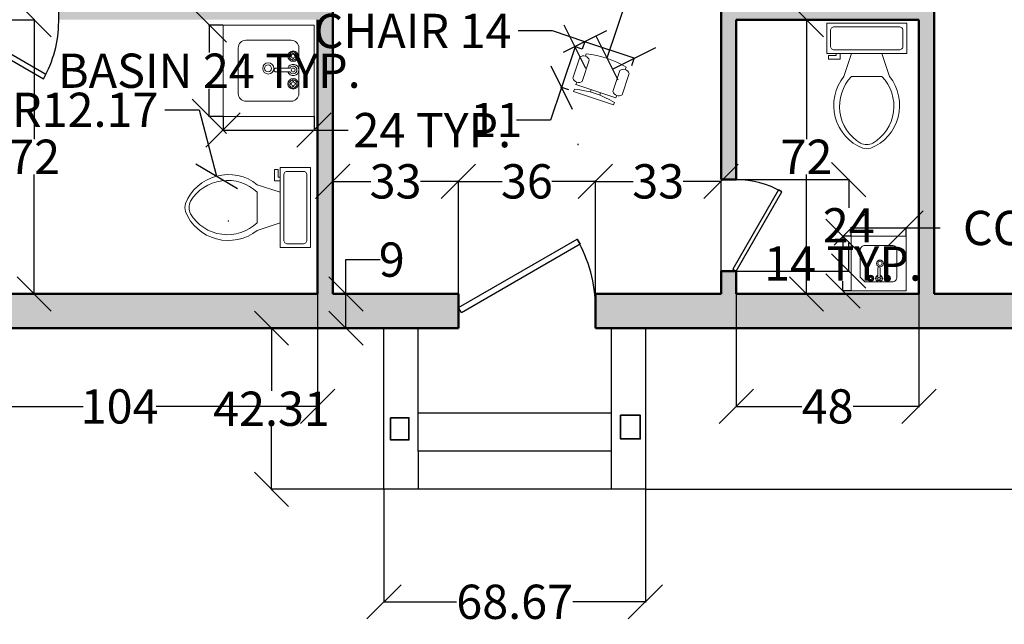
# Model space of a CAD drawing. Units: inches. Extents: x -9 to 615, y -420 to 89.
# Tile 2 of 6: x 201 to 460, y -420 to -261. Entities that reach past the tile are written whole.
import ezdxf

# ---------------------------------------------------------------- set-up
doc = ezdxf.new("R2010")
doc.units = ezdxf.units.IN
doc.header["$MEASUREMENT"] = 0
for name, color, linetype, lineweight in [('A-ANNO-DIMS', 2, 'Continuous', 18), ('A-COLS', 7, 'Continuous', 35), ('A-DOOR', 4, 'Continuous', 25), ('A-FLOR-FIXT', 9, 'Continuous', 18), ('A-FLOR-STRS', 7, 'Continuous', 25), ('A-FURN', 8, 'Continuous', 18), ('A-WALL', 7, 'Continuous', 50)]:
    doc.layers.add(name, color=color, linetype=linetype, lineweight=lineweight)
doc.layers.add('A-WALL-PATT', color=251, linetype='Continuous', lineweight=13, true_color=0x636466)
doc.styles.get("Standard").update_dxf_attribs({"font": 'arial.ttf'})
doc.dimstyles.get("Standard").update_dxf_attribs({"dimtxt": 9, "dimasz": 9, "dimexe": 0.18, "dimexo": 0.0625, "dimgap": 0.09, "dimtad": 0, "dimtih": 1, "dimtoh": 1, "dimdec": 0, "dimzin": 0, "dimdsep": 46, "dimlunit": 4, "dimtxsty": 'Standard', "dimblk": 'OBLIQUE', "dimblk2": 'OBLIQUE', "dimcen": 0.09, "dimadec": 0, "dimazin": 0, "dimtfac": 1, "dimtdec": 0, "dimtofl": 0, "dimtmove": 0, "dimatfit": 3, "dimldrblk": 'OBLIQUE', "dimfxl": 1, "dimtolj": 1, "dimtzin": 0, "dimarcsym": 0})

# ---------------------------------------------------------------- blocks, each defined once
blk = doc.blocks.new('Chair - Desk')
for p, q in [((-8.5, 0), (-8.5, -1)), ((-8.5, 0), (8.5, 0)), ((8.5, 0), (8.5, -1)), ((-8.5, -3), (-8.5, -4)), ((-8.5, -3), (8.5, -3)), ((-2, -3), (-2, -1.9355)), ((2, -1.9576), (2, -3)), ((8.5, -3), (8.5, -4)), ((-10.5, -5), (-10.5, -14)), ((-6.5, -14), (-6.5, -5)), ((6.5, -5), (6.5, -14)), ((10.5, -14), (10.5, -5)), ((-8.5, -15), (-8.5, -16)), ((8.5, -15), (8.5, -16))]:
    blk.add_line(p, q)
for centre, radius, start, end in [((0, 34.625), 36.625, 256.5803, 283.4197), ((-8.5, -6.5), 2.5, 36.8699, 143.1301), ((8.5, -6.5), 2.5, 36.8699, 143.1301), ((-8.5, -12.5), 2.5, 216.8699, 323.1301), ((8.5, -12.5), 2.5, 216.8699, 323.1301), ((0, 19.625), 36.625, 256.5803, 283.4197)]:
    blk.add_arc(centre, radius, start, end)
blk = doc.blocks.new('Toilet - top')
for p, q in [((9.5, -6), (9.5, -2)), ((-10, -8.5), (-8, -8.5)), ((-10, -9.5), (-10, -8.5)), ((-7, -9.5), (-10, -9.5)), ((-8, -8.5), (-8, -8)), ((-7, -8), (-7, -9.5)), ((-4, -8), (-6, -14)), ((4, -8), (6, -14)), ((4, -14), (-4, -14))]:
    blk.add_line(p, q)
blk.add_lwpolyline([(10.5, -8), (10.5, 0), (-10.5, 0), (-10.5, -8)], close=True)
for points in [[(-9.5, -2), (-9.5, -6)], [(8.5, -1), (-8.5, -1)], [(-8.5, -7), (8.5, -7)]]:
    blk.add_lwpolyline(points)
for centre, radius, start, end in [((-8.62, -1.88), 0.884, 81.8699, 188.1301), ((8.62, -1.88), 0.884, 351.8699, 98.1301), ((-8.62, -6.12), 0.884, 171.8699, 278.1301), ((8.62, -6.12), 0.884, 261.8699, 8.1301), ((3.52, -21.58), 12.17, 141.4691, 247.9714), ((4.2, -21.82), 11.33, 136.3677, 238.9468), ((-3.52, -21.58), 12.17, 292.0284, 38.5307), ((-4.2, -21.82), 11.33, 301.053, 43.6321), ((0, -27.88), 4, 245.7318, 294.2682), ((0, -29), 4, 254.8605, 285.1395)]:
    blk.add_arc(centre, radius, start, end)
blk = doc.blocks.new('*U12')
for p, q in [((0, 0), (0, -6)), ((40, 0), (40, -6))]:
    blk.add_line(p, q)
blk.add_lwpolyline([(0, 0), (34.64, 20), (35.52, 18.48), (0.87, -1.52)], close=True)
blk.add_arc((0, 0), 40, 0, 30)
blk = doc.blocks.new('*U13')
for p, q in [((0, 0), (0, 6)), ((40, 0), (40, 6))]:
    blk.add_line(p, q)
blk.add_lwpolyline([(0, 0), (34.64, -20), (35.52, -18.48), (0.87, 1.52)], close=True)
blk.add_arc((0, 0), 40, 330, 0)
blk = doc.blocks.new('Faucet - Bathroom top')
for p, q in [((-4.107, 0.125), (-4.375, 0.125)), ((-3.75, 0.4788), (-3.75, 0.75)), ((-3.5, 0.482), (-3.5, 0.75)), ((-3.1461, 0.125), (-2.875, 0.125)), ((3.143, 0.125), (2.875, 0.125)), ((3.5, 0.4788), (3.5, 0.75)), ((3.75, 0.482), (3.75, 0.75)), ((4.1039, 0.125), (4.375, 0.125)), ((-4.1039, -0.125), (-4.375, -0.125)), ((-3.75, -0.4821), (-3.75, -0.75)), ((-3.5, -0.4789), (-3.5, -0.75)), ((-3.143, -0.125), (-2.875, -0.125)), ((-0.5, -0.8639), (-0.5, -4.5)), ((0.5, -4.5), (0.5, -0.8631)), ((3.1461, -0.125), (2.875, -0.125)), ((3.5, -0.4821), (3.5, -0.75)), ((3.75, -0.4789), (3.75, -0.75)), ((4.107, -0.125), (4.375, -0.125))]:
    blk.add_line(p, q)
for centre, radius in [((-3.625, 0), 1.375), ((-4.625, 0), 0.2795), ((-3.625, 0), 0.5), ((-3.625, 1), 0.2795), ((-2.625, 0), 0.2795), ((0, 0), 0.5), ((3.625, 0), 1.375), ((2.625, 0), 0.2795), ((3.625, 0), 0.5), ((3.625, 1), 0.2795), ((4.625, 0), 0.2795), ((-3.625, -1), 0.2795), ((3.625, -1), 0.2795)]:
    blk.add_circle(centre, radius)
for centre, radius, start, end in [((-3.625, 0), 1, 105.2407, 164.2093), ((-3.625, 0), 1, 16.44125, 74.07887), ((0, 0), 1.5, 289.6514, 250.3603), ((0, 0), 1, 300.3431, 239.7554), ((3.625, 0), 1, 106.12, 164.0884), ((3.625, 0), 1, 16.23422, 73.90469), ((-3.625, 0), 1, 196.2342, 253.9047), ((-3.625, 0), 1, 286.12, 344.0884), ((3.625, 0), 1, 196.4413, 254.0789), ((3.625, 0), 1, 285.2407, 344.2093), ((0, -4.5), 0.5, 180, 0)]:
    blk.add_arc(centre, radius, start, end)
blk = doc.blocks.new('LAVATORY-24IN')
blk.add_lwpolyline([(0, 23.91), (0, 0), (24, 0), (24, 23.91)], close=True)
blk.add_lwpolyline([(4, 17.91), (4, 6, 0.414214), (6, 4), (18, 4, 0.414214), (20, 6), (20, 17.91, 0.414214), (18, 19.91), (6, 19.91, 0.414214)], format="xyb", close=True)
for centre, radius in [((11.41, 11.89), 1.47), ((11.39, 11.82), 0.91)]:
    blk.add_circle(centre, radius)
blk.add_blockref('Faucet - Bathroom top', (11.81, 18.42))
blk = doc.blocks.new('LAVATORY-COMPACT')
blk.add_lwpolyline([(14.42, 0), (14.42, 14.37), (0, 14.37), (0, 0)], close=True)
blk.add_lwpolyline([(12.02, 3.61), (12.02, 10.76, 0.414214), (10.82, 11.96), (3.61, 11.96, 0.414214), (2.4, 10.76), (2.4, 3.61), (3.61, 2.4), (10.82, 2.4, 0.414214)], format="xyb", close=True)
for centre, radius in [((7.57, 7.22), 0.886), ((7.57, 7.26), 0.547)]:
    blk.add_circle(centre, radius)
at = {"xscale": 0.6009252125773316, "yscale": 0.6009252125773316, "zscale": 0.6009252125773316, "rotation": 180}
blk.add_blockref('Faucet - Bathroom top', (7.32, 3.3), dxfattribs=at)
blk = doc.blocks.new('_Oblique')
at = {"color": 0, "linetype": 'ByBlock', "lineweight": -2}
blk.add_line((-0.5, -0.5), (0.5, 0.5), dxfattribs=at)
blk = doc.blocks.new('*D22')
at = {"layer": 'A-ANNO-DIMS', "color": 0, "lineweight": -2, "transparency": 16777216}
for p, q in [((254.55, -262.38), (250.83, -262.38)), ((251.01, -262.38), (251.01, -269.63)), ((251.01, -286.38), (251.01, -279.12)), ((254.55, -286.38), (250.83, -286.38))]:
    blk.add_line(p, q, dxfattribs=at)
at = {"layer": 'Defpoints', "color": 0, "transparency": 16777216}
for p in [(254.61, -262.38), (251.01, -286.38), (254.61, -286.38)]:
    blk.add_point(p, dxfattribs=at)
at = {"layer": 'A-ANNO-DIMS', "color": 0, "lineweight": -2, "transparency": 16777216, "xscale": 9, "yscale": 9, "zscale": 9}
for p, rotation in [((251.01, -262.38), 90), ((251.01, -286.38), 270)]:
    blk.add_blockref('_Oblique', p, dxfattribs=dict(at, rotation=rotation))
at = {"layer": 'A-ANNO-DIMS', "color": 0, "transparency": 16777216, "insert": (251.01, -274.38), "char_height": 9, "attachment_point": 5}
blk.add_mtext('\\A1;BASIN 24 TYP.', dxfattribs=at)
blk = doc.blocks.new('*D23')
at = {"layer": 'A-ANNO-DIMS', "color": 0, "lineweight": -2, "transparency": 16777216}
for p, q in [((254.61, -286.44), (254.61, -290.16)), ((278.52, -286.44), (278.52, -290.16)), ((254.61, -289.98), (278.52, -289.98)), ((278.52, -289.98), (287.52, -289.98))]:
    blk.add_line(p, q, dxfattribs=at)
at = {"layer": 'Defpoints', "color": 0, "transparency": 16777216}
for p in [(254.61, -286.38), (278.52, -286.38), (278.52, -289.98)]:
    blk.add_point(p, dxfattribs=at)
at = {"layer": 'A-ANNO-DIMS', "color": 0, "lineweight": -2, "transparency": 16777216, "xscale": 9, "yscale": 9, "zscale": 9, "rotation": 180}
blk.add_blockref('_Oblique', (254.61, -289.98), dxfattribs=at)
at = {"layer": 'A-ANNO-DIMS', "color": 0, "lineweight": -2, "transparency": 16777216, "xscale": 9, "yscale": 9, "zscale": 9}
blk.add_blockref('_Oblique', (278.52, -289.98), dxfattribs=at)
at = {"layer": 'A-ANNO-DIMS', "color": 0, "transparency": 16777216, "insert": (309.59, -289.98), "char_height": 9, "attachment_point": 5}
blk.add_mtext('\\A1;24 TYP.', dxfattribs=at)
blk = doc.blocks.new('*D24')
at = {"layer": 'A-ANNO-DIMS', "color": 0, "lineweight": -2, "transparency": 16777216}
for p, q in [((419.63, -317.77), (419.63, -315.49)), ((434.05, -317.77), (434.05, -315.49)), ((419.63, -315.67), (434.05, -315.67)), ((434.05, -315.67), (443.05, -315.67))]:
    blk.add_line(p, q, dxfattribs=at)
at = {"layer": 'Defpoints', "color": 0, "transparency": 16777216}
for p in [(419.63, -317.84), (434.05, -315.67), (434.05, -317.84)]:
    blk.add_point(p, dxfattribs=at)
at = {"layer": 'A-ANNO-DIMS', "color": 0, "lineweight": -2, "transparency": 16777216, "xscale": 9, "yscale": 9, "zscale": 9, "rotation": 180}
blk.add_blockref('_Oblique', (419.63, -315.67), dxfattribs=at)
at = {"layer": 'A-ANNO-DIMS', "color": 0, "lineweight": -2, "transparency": 16777216, "xscale": 9, "yscale": 9, "zscale": 9}
blk.add_blockref('_Oblique', (434.05, -315.67), dxfattribs=at)
at = {"layer": 'A-ANNO-DIMS', "color": 0, "transparency": 16777216, "insert": (518.79, -315.67), "char_height": 9, "attachment_point": 5}
blk.add_mtext('\\A1;COMPACT BASIN 14 TYP.', dxfattribs=at)
blk = doc.blocks.new('*D25')
at = {"layer": 'A-ANNO-DIMS', "color": 0, "lineweight": -2, "transparency": 16777216}
for p, q in [((419.57, -317.84), (417.29, -317.84)), ((417.47, -317.84), (417.47, -320.41)), ((417.47, -332.2), (417.47, -329.63)), ((419.57, -332.2), (417.29, -332.2))]:
    blk.add_line(p, q, dxfattribs=at)
at = {"layer": 'Defpoints', "color": 0, "transparency": 16777216}
for p in [(417.47, -317.84), (419.63, -317.84), (419.63, -332.2)]:
    blk.add_point(p, dxfattribs=at)
at = {"layer": 'A-ANNO-DIMS', "color": 0, "lineweight": -2, "transparency": 16777216, "xscale": 9, "yscale": 9, "zscale": 9}
for p, rotation in [((417.47, -317.84), 90), ((417.47, -332.2), 270)]:
    blk.add_blockref('_Oblique', p, dxfattribs=dict(at, rotation=rotation))
at = {"layer": 'A-ANNO-DIMS', "color": 0, "transparency": 16777216, "insert": (417.47, -325.02), "char_height": 9, "attachment_point": 5}
blk.add_mtext('\\A1;14 TYP.', dxfattribs=at)
blk = doc.blocks.new('*D30')
at = {"layer": 'A-ANNO-DIMS', "color": 0, "lineweight": -2, "transparency": 16777216}
for p, q in [((341.16, -263.93), (332.16, -263.93)), ((349.7, -266.78), (341.16, -263.93)), ((349.07, -268.67), (349.75, -266.61)), ((362.66, -271.11), (349.7, -266.78)), ((362.03, -272.99), (362.72, -270.94))]:
    blk.add_line(p, q, dxfattribs=at)
at = {"layer": 'Defpoints', "color": 0, "transparency": 16777216}
for p in [(349.05, -268.73), (349.7, -266.78), (362.01, -273.05)]:
    blk.add_point(p, dxfattribs=at)
at = {"layer": 'A-ANNO-DIMS', "color": 0, "lineweight": -2, "transparency": 16777216, "xscale": 9, "yscale": 9, "zscale": 9}
for p, rotation in [((349.7, -266.78), 161.5484668350482), ((362.66, -271.11), 341.5484668350483)]:
    blk.add_blockref('_Oblique', p, dxfattribs=dict(at, rotation=rotation))
at = {"layer": 'A-ANNO-DIMS', "color": 0, "transparency": 16777216, "insert": (304.39, -263.93), "char_height": 9, "attachment_point": 5}
blk.add_mtext('\\A1;CHAIR 14', dxfattribs=at)
blk = doc.blocks.new('*D31')
at = {"layer": 'A-ANNO-DIMS', "color": 0, "lineweight": -2, "transparency": 16777216}
for p, q in [((347.1, -268.08), (343.53, -278.78)), ((348.99, -268.71), (346.93, -268.02)), ((343.53, -278.78), (340.68, -287.32)), ((345.42, -279.41), (343.36, -278.72)), ((340.68, -287.32), (331.68, -287.32))]:
    blk.add_line(p, q, dxfattribs=at)
at = {"layer": 'Defpoints', "color": 0, "transparency": 16777216}
for p in [(349.05, -268.73), (343.53, -278.78), (345.48, -279.43)]:
    blk.add_point(p, dxfattribs=at)
at = {"layer": 'A-ANNO-DIMS', "color": 0, "lineweight": -2, "transparency": 16777216, "xscale": 9, "yscale": 9, "zscale": 9}
for p, rotation in [((347.1, -268.08), 71.54846683504834), ((343.53, -278.78), 251.5484668350484)]:
    blk.add_blockref('_Oblique', p, dxfattribs=dict(at, rotation=rotation))
at = {"layer": 'A-ANNO-DIMS', "color": 0, "transparency": 16777216, "insert": (326.44, -287.32), "char_height": 9, "attachment_point": 5}
blk.add_mtext('\\A1;11', dxfattribs=at)
blk = doc.blocks.new('*D42')
at = {"layer": 'A-ANNO-DIMS', "color": 0, "lineweight": -2, "transparency": 16777216}
for p, q in [((437.5, 54.02), (600.17, 54.02)), ((599.99, 54.02), (599.99, -160.45)), ((599.99, -384.29), (599.99, -169.82)), ((365.62, -384.29), (600.17, -384.29))]:
    blk.add_line(p, q, dxfattribs=at)
at = {"layer": 'Defpoints', "color": 0, "transparency": 16777216}
for p in [(437.44, 54.02), (599.99, 54.02), (365.56, -384.29)]:
    blk.add_point(p, dxfattribs=at)
at = {"layer": 'A-ANNO-DIMS', "color": 0, "lineweight": -2, "transparency": 16777216, "xscale": 9, "yscale": 9, "zscale": 9}
for p, rotation in [((599.99, 54.02), 90), ((599.99, -384.29), 270)]:
    blk.add_blockref('_Oblique', p, dxfattribs=dict(at, rotation=rotation))
at = {"layer": 'A-ANNO-DIMS', "color": 0, "transparency": 16777216, "insert": (599.99, -165.14), "char_height": 9, "attachment_point": 5}
blk.add_mtext('\\A1;438.3', dxfattribs=at)
blk = doc.blocks.new('*D50')
at = {"layer": 'A-ANNO-DIMS', "color": 0, "lineweight": -2, "transparency": 16777216}
for p, q in [((175.44, -333.04), (175.44, -362.71)), ((279.44, -333.04), (279.44, -362.71)), ((175.44, -362.53), (217.85, -362.53)), ((279.44, -362.53), (237.03, -362.53))]:
    blk.add_line(p, q, dxfattribs=at)
at = {"layer": 'Defpoints', "color": 0, "transparency": 16777216}
for p in [(175.44, -332.98), (279.44, -332.98), (175.44, -362.53)]:
    blk.add_point(p, dxfattribs=at)
at = {"layer": 'A-ANNO-DIMS', "color": 0, "lineweight": -2, "transparency": 16777216, "xscale": 9, "yscale": 9, "zscale": 9, "rotation": 180}
blk.add_blockref('_Oblique', (175.44, -362.53), dxfattribs=at)
at = {"layer": 'A-ANNO-DIMS', "color": 0, "lineweight": -2, "transparency": 16777216, "xscale": 9, "yscale": 9, "zscale": 9}
blk.add_blockref('_Oblique', (279.44, -362.53), dxfattribs=at)
at = {"layer": 'A-ANNO-DIMS', "color": 0, "transparency": 16777216, "insert": (227.44, -362.53), "char_height": 9, "attachment_point": 5}
blk.add_mtext('\\A1;104', dxfattribs=at)
blk = doc.blocks.new('*D51')
at = {"layer": 'A-ANNO-DIMS', "color": 0, "lineweight": -2, "transparency": 16777216}
for p, q in [((283.44, -332.92), (283.44, -303.25)), ((283.44, -303.43), (293.4, -303.43)), ((316.44, -303.43), (306.47, -303.43)), ((316.44, -332.92), (316.44, -303.25))]:
    blk.add_line(p, q, dxfattribs=at)
at = {"layer": 'Defpoints', "color": 0, "transparency": 16777216}
for p in [(316.44, -303.43), (283.44, -332.98), (316.44, -332.98)]:
    blk.add_point(p, dxfattribs=at)
at = {"layer": 'A-ANNO-DIMS', "color": 0, "lineweight": -2, "transparency": 16777216, "xscale": 9, "yscale": 9, "zscale": 9, "rotation": 180}
blk.add_blockref('_Oblique', (283.44, -303.43), dxfattribs=at)
at = {"layer": 'A-ANNO-DIMS', "color": 0, "lineweight": -2, "transparency": 16777216, "xscale": 9, "yscale": 9, "zscale": 9}
blk.add_blockref('_Oblique', (316.44, -303.43), dxfattribs=at)
at = {"layer": 'A-ANNO-DIMS', "color": 0, "transparency": 16777216, "insert": (299.94, -303.43), "char_height": 9, "attachment_point": 5}
blk.add_mtext('\\A1;33', dxfattribs=at)
blk = doc.blocks.new('*D52')
at = {"layer": 'A-ANNO-DIMS', "color": 0, "lineweight": -2, "transparency": 16777216}
for p, q in [((316.44, -332.92), (316.44, -303.25)), ((316.44, -303.43), (327.91, -303.43)), ((352.44, -303.43), (340.97, -303.43)), ((352.44, -332.92), (352.44, -303.25))]:
    blk.add_line(p, q, dxfattribs=at)
at = {"layer": 'Defpoints', "color": 0, "transparency": 16777216}
for p in [(352.44, -303.43), (316.44, -332.98), (352.44, -332.98)]:
    blk.add_point(p, dxfattribs=at)
at = {"layer": 'A-ANNO-DIMS', "color": 0, "lineweight": -2, "transparency": 16777216, "xscale": 9, "yscale": 9, "zscale": 9, "rotation": 180}
blk.add_blockref('_Oblique', (316.44, -303.43), dxfattribs=at)
at = {"layer": 'A-ANNO-DIMS', "color": 0, "lineweight": -2, "transparency": 16777216, "xscale": 9, "yscale": 9, "zscale": 9}
blk.add_blockref('_Oblique', (352.44, -303.43), dxfattribs=at)
at = {"layer": 'A-ANNO-DIMS', "color": 0, "transparency": 16777216, "insert": (334.44, -303.43), "char_height": 9, "attachment_point": 5}
blk.add_mtext('\\A1;36', dxfattribs=at)
blk = doc.blocks.new('*D53')
at = {"layer": 'A-ANNO-DIMS', "color": 0, "lineweight": -2, "transparency": 16777216}
for p, q in [((352.44, -332.92), (352.44, -303.25)), ((352.44, -303.43), (362.4, -303.43)), ((385.44, -303.43), (375.47, -303.43)), ((385.44, -332.92), (385.44, -303.25))]:
    blk.add_line(p, q, dxfattribs=at)
at = {"layer": 'Defpoints', "color": 0, "transparency": 16777216}
for p in [(385.44, -303.43), (352.44, -332.98), (385.44, -332.98)]:
    blk.add_point(p, dxfattribs=at)
at = {"layer": 'A-ANNO-DIMS', "color": 0, "lineweight": -2, "transparency": 16777216, "xscale": 9, "yscale": 9, "zscale": 9, "rotation": 180}
blk.add_blockref('_Oblique', (352.44, -303.43), dxfattribs=at)
at = {"layer": 'A-ANNO-DIMS', "color": 0, "lineweight": -2, "transparency": 16777216, "xscale": 9, "yscale": 9, "zscale": 9}
blk.add_blockref('_Oblique', (385.44, -303.43), dxfattribs=at)
at = {"layer": 'A-ANNO-DIMS', "color": 0, "transparency": 16777216, "insert": (368.94, -303.43), "char_height": 9, "attachment_point": 5}
blk.add_mtext('\\A1;33', dxfattribs=at)
blk = doc.blocks.new('*D54')
at = {"layer": 'A-ANNO-DIMS', "color": 0, "lineweight": -2, "transparency": 16777216}
for p, q in [((389.44, -333.04), (389.44, -362.71)), ((437.44, -333.04), (437.44, -362.71)), ((389.44, -362.53), (406.71, -362.53)), ((437.44, -362.53), (420.16, -362.53))]:
    blk.add_line(p, q, dxfattribs=at)
at = {"layer": 'Defpoints', "color": 0, "transparency": 16777216}
for p in [(389.44, -332.98), (437.44, -332.98), (389.44, -362.53)]:
    blk.add_point(p, dxfattribs=at)
at = {"layer": 'A-ANNO-DIMS', "color": 0, "lineweight": -2, "transparency": 16777216, "xscale": 9, "yscale": 9, "zscale": 9, "rotation": 180}
blk.add_blockref('_Oblique', (389.44, -362.53), dxfattribs=at)
at = {"layer": 'A-ANNO-DIMS', "color": 0, "lineweight": -2, "transparency": 16777216, "xscale": 9, "yscale": 9, "zscale": 9}
blk.add_blockref('_Oblique', (437.44, -362.53), dxfattribs=at)
at = {"layer": 'A-ANNO-DIMS', "color": 0, "transparency": 16777216, "insert": (413.44, -362.53), "char_height": 9, "attachment_point": 5}
blk.add_mtext('\\A1;48', dxfattribs=at)
blk = doc.blocks.new('*D62')
at = {"layer": 'A-ANNO-DIMS', "color": 0, "lineweight": -2, "transparency": 16777216}
for p, q in [((175.5, -260.98), (205.17, -260.98)), ((204.99, -260.98), (204.99, -292.37)), ((204.99, -332.98), (204.99, -301.59)), ((175.5, -332.98), (205.17, -332.98))]:
    blk.add_line(p, q, dxfattribs=at)
at = {"layer": 'Defpoints', "color": 0, "transparency": 16777216}
for p in [(175.44, -260.98), (175.44, -332.98), (204.99, -332.98)]:
    blk.add_point(p, dxfattribs=at)
at = {"layer": 'A-ANNO-DIMS', "color": 0, "lineweight": -2, "transparency": 16777216, "xscale": 9, "yscale": 9, "zscale": 9}
for p, rotation in [((204.99, -260.98), 90), ((204.99, -332.98), 270)]:
    blk.add_blockref('_Oblique', p, dxfattribs=dict(at, rotation=rotation))
at = {"layer": 'A-ANNO-DIMS', "color": 0, "transparency": 16777216, "insert": (204.99, -296.98), "char_height": 9, "attachment_point": 5}
blk.add_mtext('\\A1;72', dxfattribs=at)
blk = doc.blocks.new('*D63')
at = {"layer": 'A-ANNO-DIMS', "color": 0, "lineweight": -2, "transparency": 16777216}
for p, q in [((437.38, -260.98), (407.71, -260.98)), ((407.89, -260.98), (407.89, -292.37)), ((407.89, -332.98), (407.89, -301.59)), ((437.38, -332.98), (407.71, -332.98))]:
    blk.add_line(p, q, dxfattribs=at)
at = {"layer": 'Defpoints', "color": 0, "transparency": 16777216}
for p in [(407.89, -260.98), (437.44, -260.98), (437.44, -332.98)]:
    blk.add_point(p, dxfattribs=at)
at = {"layer": 'A-ANNO-DIMS', "color": 0, "lineweight": -2, "transparency": 16777216, "xscale": 9, "yscale": 9, "zscale": 9}
for p, rotation in [((407.89, -260.98), 90), ((407.89, -332.98), 270)]:
    blk.add_blockref('_Oblique', p, dxfattribs=dict(at, rotation=rotation))
at = {"layer": 'A-ANNO-DIMS', "color": 0, "transparency": 16777216, "insert": (407.89, -296.98), "char_height": 9, "attachment_point": 5}
blk.add_mtext('\\A1;72', dxfattribs=at)
blk = doc.blocks.new('*D65')
at = {"layer": 'A-ANNO-DIMS', "color": 0, "lineweight": -2, "transparency": 16777216}
for p, q in [((286.89, -332.98), (286.89, -323.98)), ((286.89, -323.98), (295.89, -323.98)), ((316.38, -332.98), (286.71, -332.98)), ((286.89, -341.98), (286.89, -332.98)), ((316.38, -341.98), (286.71, -341.98))]:
    blk.add_line(p, q, dxfattribs=at)
at = {"layer": 'Defpoints', "color": 0, "transparency": 16777216}
for p in [(286.89, -332.98), (316.44, -332.98), (316.44, -341.98)]:
    blk.add_point(p, dxfattribs=at)
at = {"layer": 'A-ANNO-DIMS', "color": 0, "lineweight": -2, "transparency": 16777216, "xscale": 9, "yscale": 9, "zscale": 9}
for p, rotation in [((286.89, -332.98), 90), ((286.89, -341.98), 270)]:
    blk.add_blockref('_Oblique', p, dxfattribs=dict(at, rotation=rotation))
at = {"layer": 'A-ANNO-DIMS', "color": 0, "transparency": 16777216, "insert": (298.94, -323.98), "char_height": 9, "attachment_point": 5}
blk.add_mtext('\\A1;9', dxfattribs=at)
blk = doc.blocks.new('*D72')
at = {"layer": 'A-ANNO-DIMS', "color": 0, "lineweight": -2, "transparency": 16777216}
for p, q in [((296.83, -341.98), (267.16, -341.98)), ((267.34, -341.98), (267.34, -358.45)), ((267.34, -384.29), (267.34, -367.82)), ((296.83, -384.29), (267.16, -384.29))]:
    blk.add_line(p, q, dxfattribs=at)
at = {"layer": 'Defpoints', "color": 0, "transparency": 16777216}
for p in [(267.34, -341.98), (296.89, -341.98), (296.89, -384.29)]:
    blk.add_point(p, dxfattribs=at)
at = {"layer": 'A-ANNO-DIMS', "color": 0, "lineweight": -2, "transparency": 16777216, "xscale": 9, "yscale": 9, "zscale": 9}
for p, rotation in [((267.34, -341.98), 90), ((267.34, -384.29), 270)]:
    blk.add_blockref('_Oblique', p, dxfattribs=dict(at, rotation=rotation))
at = {"layer": 'A-ANNO-DIMS', "color": 0, "transparency": 16777216, "insert": (267.34, -363.14), "char_height": 9, "attachment_point": 5}
blk.add_mtext('\\A1;42.31', dxfattribs=at)
blk = doc.blocks.new('*D73')
at = {"layer": 'A-ANNO-DIMS', "color": 0, "lineweight": -2, "transparency": 16777216}
for p, q in [((296.89, -384.35), (296.89, -414.02)), ((365.56, -384.35), (365.56, -414.02)), ((296.89, -413.84), (315.93, -413.84)), ((365.56, -413.84), (346.52, -413.84))]:
    blk.add_line(p, q, dxfattribs=at)
at = {"layer": 'Defpoints', "color": 0, "transparency": 16777216}
for p in [(296.89, -384.29), (365.56, -384.29), (296.89, -413.84)]:
    blk.add_point(p, dxfattribs=at)
at = {"layer": 'A-ANNO-DIMS', "color": 0, "lineweight": -2, "transparency": 16777216, "xscale": 9, "yscale": 9, "zscale": 9, "rotation": 180}
blk.add_blockref('_Oblique', (296.89, -413.84), dxfattribs=at)
at = {"layer": 'A-ANNO-DIMS', "color": 0, "lineweight": -2, "transparency": 16777216, "xscale": 9, "yscale": 9, "zscale": 9}
blk.add_blockref('_Oblique', (365.56, -413.84), dxfattribs=at)
at = {"layer": 'A-ANNO-DIMS', "color": 0, "transparency": 16777216, "insert": (331.23, -413.84), "char_height": 9, "attachment_point": 5}
blk.add_mtext('\\A1;68.67', dxfattribs=at)
blk = doc.blocks.new('*D86')
at = {"layer": 'A-ANNO-DIMS', "color": 0, "lineweight": -2, "transparency": 16777216}
for p, q in [((389.5, -302.98), (419.17, -302.98)), ((418.99, -302.98), (418.99, -310.37)), ((418.99, -326.98), (418.99, -319.59)), ((389.5, -326.98), (419.17, -326.98))]:
    blk.add_line(p, q, dxfattribs=at)
at = {"layer": 'Defpoints', "color": 0, "transparency": 16777216}
for p in [(389.44, -302.98), (389.44, -326.98), (418.99, -326.98)]:
    blk.add_point(p, dxfattribs=at)
at = {"layer": 'A-ANNO-DIMS', "color": 0, "lineweight": -2, "transparency": 16777216, "xscale": 9, "yscale": 9, "zscale": 9}
for p, rotation in [((418.99, -302.98), 90), ((418.99, -326.98), 270)]:
    blk.add_blockref('_Oblique', p, dxfattribs=dict(at, rotation=rotation))
at = {"layer": 'A-ANNO-DIMS', "color": 0, "transparency": 16777216, "insert": (418.99, -314.98), "char_height": 9, "attachment_point": 5}
blk.add_mtext('\\A1;24', dxfattribs=at)
blk = doc.blocks.new('*D92')
at = {"layer": 'A-ANNO-DIMS', "color": 0, "lineweight": -2, "transparency": 16777216}
for p, q in [((239.35, -284.65), (248.35, -284.65)), ((248.35, -284.65), (252.92, -302.06)), ((255.92, -313.83), (256.1, -313.83)), ((256.01, -313.92), (256.01, -313.74))]:
    blk.add_line(p, q, dxfattribs=at)
at = {"layer": 'Defpoints', "color": 0, "transparency": 16777216}
for p in [(252.92, -302.06), (256.01, -313.83)]:
    blk.add_point(p, dxfattribs=at)
at = {"layer": 'A-ANNO-DIMS', "color": 0, "lineweight": -2, "transparency": 16777216, "xscale": 9, "yscale": 9, "zscale": 9, "rotation": 284.7182478829065}
blk.add_blockref('_Oblique', (252.92, -302.06), dxfattribs=at)
at = {"layer": 'A-ANNO-DIMS', "color": 0, "transparency": 16777216, "insert": (210.09, -284.65), "char_height": 9, "attachment_point": 5}
blk.add_mtext('\\A1;8X R12.17', dxfattribs=at)
blk = doc.blocks.new('*D94')
at = {"layer": 'A-ANNO-DIMS', "color": 0, "lineweight": -2, "transparency": 16777216}
for p, q in [((361.16, -254.02), (355.46, -271.1)), ((370.16, -254.02), (361.16, -254.02)), ((347.83, -293.71), (348.01, -293.71)), ((347.92, -293.8), (347.92, -293.62))]:
    blk.add_line(p, q, dxfattribs=at)
at = {"layer": 'Defpoints', "color": 0, "transparency": 16777216}
for p in [(355.46, -271.1), (347.92, -293.71)]:
    blk.add_point(p, dxfattribs=at)
at = {"layer": 'A-ANNO-DIMS', "color": 0, "lineweight": -2, "transparency": 16777216, "xscale": 9, "yscale": 9, "zscale": 9, "rotation": 251.5488985370354}
blk.add_blockref('_Oblique', (355.46, -271.1), dxfattribs=at)
at = {"layer": 'A-ANNO-DIMS', "color": 0, "transparency": 16777216, "insert": (399.47, -254.02), "char_height": 9, "attachment_point": 5}
blk.add_mtext('\\A1;2X R23.84', dxfattribs=at)

msp = doc.modelspace()

# ---------------------------------------------------------------- hatches: boundary and pattern name
at = {"layer": 'A-WALL-PATT'}
h = msp.add_hatch(color=256, dxfattribs=at)
h.dxf.hatch_style = 1
h.paths.add_polyline_path([(389.4378, 18.0183), (30.4378, 18.0183), (30.4378, -341.9817), (316.4378, -341.9817), (316.4378, -336.5817), (316.4378, -332.9817), (283.4378, -332.9817), (283.4378, -256.9817), (283.4378, -250.9817), (283.4378, -248.9817), (278.9378, -248.9817), (277.4378, -248.9817), (277.4378, -250.9817), (277.4378, -256.9817), (211.4378, -256.9817), (211.4378, -260.9817), (279.4378, -260.9817), (279.4378, -332.9817), (175.4378, -332.9817), (175.4378, -260.9817), (181.4378, -260.9817), (181.4378, -256.9817), (175.4378, -256.9817), (175.4378, -248.9817), (171.4378, -248.9817), (171.4378, -332.9817), (39.4378, -332.9817), (39.4378, -212.9817), (171.4378, -212.9817), (171.4378, -218.9817), (175.4378, -218.9817), (175.4378, -212.9817), (179.4378, -212.9817), (179.4378, -208.9817), (135.4378, -208.9817), (135.4378, -114.9817), (179.4378, -114.9817), (179.4378, -110.9817), (100.4378, -110.9817), (100.4378, -114.9817), (131.4378, -114.9817), (131.4378, -208.9817), (39.4378, -208.9817), (39.4378, -114.9817), (70.4378, -114.9817), (70.4378, -110.9817), (39.4378, -110.9817), (39.4378, 9.0183), (215.4378, 9.0183), (215.4378, -110.9817), (215.4378, -208.9817), (209.4378, -208.9817), (209.4378, -212.9817), (215.4378, -212.9817), (255.4378, -212.9817), (277.4378, -212.9817), (277.4378, -218.9817), (283.4378, -218.9817), (283.4378, -212.9817), (283.4378, -208.9817), (283.4378, -202.9817), (279.4378, -202.9817), (279.4378, -208.9817), (255.4378, -208.9817), (219.4378, -208.9817), (219.4378, -170.1983), (255.4378, -170.1983), (277.4378, -170.1983), (277.4378, -176.1983), (283.4378, -176.1983), (283.4378, -170.1983), (283.4378, -166.1983), (255.4378, -166.1983), (219.4378, -166.1983), (219.4378, -42.9817), (243.4378, -42.9817), (243.4378, -38.9817), (219.4378, -38.9817), (219.4378, 9.0183), (267.4378, 9.0183), (267.4378, -38.9817), (261.4378, -38.9817), (261.4378, -42.9817), (271.4378, -42.9817), (271.4378, 9.0183), (380.4378, 9.0183), (380.4378, -14.9817), (380.4378, -23.9817), (401.4378, -23.9817), (401.4378, -14.9817), (389.4378, -14.9817)])
h = msp.add_hatch(color=256, dxfattribs=at)
h.dxf.hatch_style = 1
h.paths.add_polyline_path([(570.4378, 18.0183), (437.4378, 18.0183), (437.4378, -14.9817), (437.4378, -110.9817), (385.4378, -110.9817), (385.4378, -114.9817), (385.4378, -120.9817), (389.4378, -120.9817), (389.4378, -114.9817), (437.4378, -114.9817), (447.4378, -114.9817), (447.4378, -110.9817), (441.4378, -110.9817), (441.4378, 9.0183), (561.4378, 9.0183), (561.4378, -110.9817), (477.4378, -110.9817), (477.4378, -114.9817), (497.4378, -114.9817), (497.4378, -168.9817), (501.4378, -168.9817), (501.4378, -114.9817), (561.4378, -114.9817), (561.4378, -198.9817), (531.4378, -198.9817), (501.4378, -198.9817), (501.4378, -192.9817), (497.4378, -192.9817), (497.4378, -198.9817), (477.4378, -198.9817), (477.4378, -202.9817), (561.4378, -202.9817), (561.4378, -332.9817), (441.4378, -332.9817), (441.4378, -202.9817), (447.4378, -202.9817), (447.4378, -198.9817), (437.4378, -198.9817), (431.4378, -198.9817), (431.4378, -202.9817), (437.4378, -202.9817), (437.4378, -256.9817), (389.4378, -256.9817), (389.4378, -202.9799), (407.5704, -202.9799), (407.4511, -198.9817), (389.4378, -198.9817), (385.4378, -198.9817), (385.4378, -302.9817), (389.4378, -302.9817), (389.4378, -260.9817), (437.4378, -260.9817), (437.4378, -332.9817), (389.4378, -332.9817), (389.4378, -326.9817), (385.4378, -326.9817), (385.4378, -332.9817), (352.4378, -332.9817), (352.4378, -341.9817), (570.4378, -341.9817)])

# ---------------------------------------------------------------- linework, layer by layer
at = {"layer": 'A-COLS'}
for points in [[(298.616, -365.4957), (303.4276, -365.4957), (303.4276, -371.339), (298.616, -371.339)], [(359.0541, -364.8614), (364.2118, -364.8614), (364.2118, -371.0742), (359.0541, -371.0742)]]:
    msp.add_lwpolyline(points, close=True, dxfattribs=at)
at = {"layer": 'A-FLOR-STRS'}
for p, q in [((296.8921, -384.2897), (296.8921, -341.9817)), ((305.8921, -374.2897), (305.8921, -341.9817)), ((356.5581, -341.9817), (356.5581, -374.2897)), ((365.5581, -341.9817), (365.5581, -384.2897)), ((356.5581, -364.2897), (305.8921, -364.2897)), ((356.5581, -374.2897), (305.8921, -374.2897)), ((305.8921, -374.2897), (305.8921, -384.2897)), ((356.5581, -374.2897), (356.5581, -384.2897)), ((365.5581, -384.2897), (296.8921, -384.2897))]:
    msp.add_line(p, q, dxfattribs=at)
at = {"layer": 'A-WALL'}
for p, q in [((385.4378, -198.9817), (385.4378, -302.9817)), ((441.4378, -202.9817), (441.4378, -332.9817)), ((283.4378, -332.9817), (283.4378, -256.9817)), ((279.4378, -332.9817), (279.4378, -260.9817)), ((437.4378, -260.9817), (389.4378, -260.9817)), ((389.4378, -260.9817), (389.4378, -302.9817)), ((437.4378, -260.9817), (437.4378, -332.9817)), ((389.4378, -302.9817), (385.4378, -302.9817)), ((389.4378, -326.9817), (385.4378, -326.9817)), ((385.4378, -326.9817), (385.4378, -332.9817)), ((389.4378, -326.9817), (389.4378, -332.9817)), ((215.4378, -332.9817), (175.4378, -332.9817)), ((279.4378, -332.9817), (175.4378, -332.9817)), ((316.4378, -332.9817), (283.4378, -332.9817)), ((316.4378, -332.9817), (316.4378, -341.9817)), ((385.4378, -332.9817), (352.4378, -332.9817)), ((352.4378, -332.9817), (352.4378, -341.9817)), ((437.4378, -332.9817), (389.4378, -332.9817)), ((561.4378, -332.9817), (441.4378, -332.9817))]:
    msp.add_line(p, q, dxfattribs=at)
for points in [[(316.4378, -341.9817), (30.4378, -341.9817), (30.4378, 18.0183), (389.4378, 18.0183)], [(437.4378, 18.0183), (570.4378, 18.0183), (570.4378, -341.9817), (352.4378, -341.9817)]]:
    msp.add_lwpolyline(points, dxfattribs=at)

# ---------------------------------------------------------------- block references
at = {"layer": 'A-DOOR'}
for name, p, xscale, yscale, zscale in [('*U13', (181.4378, -261.4817), 0.75, 0.75, 0.75), ('*U12', (316.4378, -336.5817), 0.9, 0.9, 0.9)]:
    msp.add_blockref(name, p, dxfattribs=dict(at, xscale=xscale, yscale=yscale, zscale=zscale))
at = {"layer": 'A-DOOR', "xscale": 0.6, "yscale": 0.6, "zscale": 0.6, "rotation": 90}
msp.add_blockref('*U13', (389.4378, -326.9817), dxfattribs=at)
at = {"layer": 'A-FLOR-FIXT'}
for name, p, rotation in [('LAVATORY-24IN', (254.6108, -262.3771), 269.9999999999999), ('Toilet - top', (277.5912, -310.3071), 270)]:
    msp.add_blockref(name, p, dxfattribs=dict(at, rotation=rotation))
for name, p in [('Toilet - top', (423.7136, -261.8769)), ('LAVATORY-COMPACT', (419.6321, -332.204))]:
    msp.add_blockref(name, p, dxfattribs=at)
at = {"layer": 'A-FURN', "xscale": 0.6508805716216762, "yscale": 0.6508805716216762, "zscale": 0.6508805716216762, "rotation": 161.5484668350484}
msp.add_blockref('Chair - Desk', (351.9611, -281.593), dxfattribs=at)

# ---------------------------------------------------------------- dimensions: what is measured, and where the dimension line sits
at = {"layer": 'A-ANNO-DIMS'}
for base, p1, p2, angle, override, picture, middle in [((599.9878, 54.0183), (365.5581, -384.2897), (437.4378, 54.0183), 90, {"dimdec": 1, "dimlfac": 1, "dimrnd": 0, "dimzin": 0, "dimdsep": 46, "dimlunit": 2}, '*D42', (599.9878, -165.1357)), ((204.9878, -332.9817), (175.4378, -260.9817), (175.4378, -332.9817), 270, {"dimdec": 0, "dimlfac": 1, "dimrnd": 0, "dimzin": 0, "dimdsep": 46, "dimlunit": 2}, '*D62', (204.9878, -296.9817)), ((407.8878, -260.9817), (437.4378, -332.9817), (437.4378, -260.9817), 90, {"dimdec": 0, "dimlfac": 1, "dimrnd": 0, "dimzin": 0, "dimdsep": 46, "dimlunit": 2}, '*D63', (407.8878, -296.9817)), ((343.5334, -278.781), (349.049, -268.728), (345.4782, -279.43), 251.548467, {"dimdec": 0, "dimlfac": 1, "dimrnd": 0, "dimzin": 0, "dimdsep": 46, "dimlunit": 2}, '*D31', (326.441, -287.3184)), ((418.9878, -326.9817), (389.4378, -302.9817), (389.4378, -326.9817), 270, {"dimdec": 0, "dimlfac": 1, "dimrnd": 0, "dimzin": 0, "dimdsep": 46, "dimlunit": 2}, '*D86', (418.9878, -314.9817)), ((286.8878, -332.9817), (316.4378, -341.9817), (316.4378, -332.9817), 90, {"dimdec": 0, "dimlfac": 1, "dimrnd": 0, "dimzin": 0, "dimdsep": 46, "dimlunit": 2}, '*D65', (298.9368, -323.9817)), ((175.4378, -362.5317), (279.4378, -332.9817), (175.4378, -332.9817), 180, {"dimdec": 0, "dimlfac": 1, "dimrnd": 0, "dimzin": 0, "dimdsep": 46, "dimlunit": 2}, '*D50', (227.4378, -362.5317)), ((389.4378, -362.5317), (437.4378, -332.9817), (389.4378, -332.9817), 180, {"dimdec": 0, "dimlfac": 1, "dimrnd": 0, "dimzin": 0, "dimdsep": 46, "dimlunit": 2}, '*D54', (413.4378, -362.5317)), ((267.3421, -341.9817), (296.8921, -384.2897), (296.8921, -341.9817), 90, {"dimdec": 2, "dimlfac": 1, "dimrnd": 0, "dimzin": 0, "dimdsep": 46, "dimlunit": 2}, '*D72', (267.3421, -363.1357)), ((296.8921, -413.8397), (365.5581, -384.2897), (296.8921, -384.2897), 180, {"dimdec": 2, "dimlfac": 1, "dimrnd": 0, "dimzin": 0, "dimdsep": 46, "dimlunit": 2}, '*D73', (331.2251, -413.8397))]:
    dim = msp.add_linear_dim(base=base, p1=p1, p2=p2, angle=angle, dimstyle='Standard', override=override, dxfattribs=at)
    dim.commit()
    dim.dimension.update_dxf_attribs({"geometry": picture, "text_midpoint": middle})
for center, mpoint, text, picture, middle in [((347.9183, -293.7099), (355.4631, -271.0968), '2X <>', '*D94', (399.4693, -254.0221)), ((256.0107, -313.8267), (252.919, -302.057), '8X <>', '*D92', (210.0887, -284.6476))]:
    dim = msp.add_radius_dim(center=center, mpoint=mpoint, text=text, dimstyle='Standard', override={"dimdec": 2, "dimlfac": 1, "dimrnd": 0, "dimzin": 0, "dimdsep": 46, "dimlunit": 2}, dxfattribs=at)
    dim.commit()
    dim.dimension.update_dxf_attribs({"geometry": picture, "text_midpoint": middle})
for base, p1, p2, angle, text, picture, middle in [((349.6979, -266.7831), (362.0148, -273.0541), (349.049, -268.728), 161.548467, 'CHAIR <>', '*D30', (304.3891, -263.9346)), ((251.0108, -286.3767), (254.6108, -262.3767), (254.6108, -286.3767), 270, 'BASIN <> TYP.', '*D22', (251.0108, -274.3767)), ((417.4684, -317.8368), (419.6317, -332.2042), (419.6317, -317.8368), 90, '<> TYP.', '*D25', (417.4684, -325.0205))]:
    dim = msp.add_linear_dim(base=base, p1=p1, p2=p2, angle=angle, text=text, dimstyle='Standard', override={"dimdec": 0, "dimlfac": 1, "dimrnd": 0, "dimzin": 0, "dimdsep": 46, "dimlunit": 2}, dxfattribs=at)
    dim.commit()
    dim.dimension.update_dxf_attribs({"geometry": picture, "text_midpoint": middle})
for base, p1, p2, text, picture, middle in [((278.5195, -289.9767), (254.6108, -286.3767), (278.5195, -286.3767), '<> TYP.', '*D23', (309.5907, -289.9767)), ((434.0539, -315.6735), (419.6317, -317.8368), (434.0539, -317.8368), 'COMPACT BASIN <> TYP.', '*D24', (518.7875, -315.6735))]:
    dim = msp.add_linear_dim(base=base, p1=p1, p2=p2, text=text, dimstyle='Standard', override={"dimdec": 0, "dimlfac": 1, "dimrnd": 0, "dimzin": 0, "dimdsep": 46, "dimlunit": 2}, dxfattribs=at)
    dim.commit()
    dim.dimension.update_dxf_attribs({"geometry": picture, "text_midpoint": middle})
for base, p1, p2, picture, middle in [((316.4378, -303.4317), (283.4378, -332.9817), (316.4378, -332.9817), '*D51', (299.9378, -303.4317)), ((352.4378, -303.4317), (316.4378, -332.9817), (352.4378, -332.9817), '*D52', (334.4378, -303.4317)), ((385.4378, -303.4317), (352.4378, -332.9817), (385.4378, -332.9817), '*D53', (368.9378, -303.4317))]:
    dim = msp.add_linear_dim(base=base, p1=p1, p2=p2, dimstyle='Standard', override={"dimdec": 0, "dimlfac": 1, "dimrnd": 0, "dimzin": 0, "dimdsep": 46, "dimlunit": 2}, dxfattribs=at)
    dim.commit()
    dim.dimension.update_dxf_attribs({"geometry": picture, "text_midpoint": middle})

doc.saveas('drawing.dxf')
